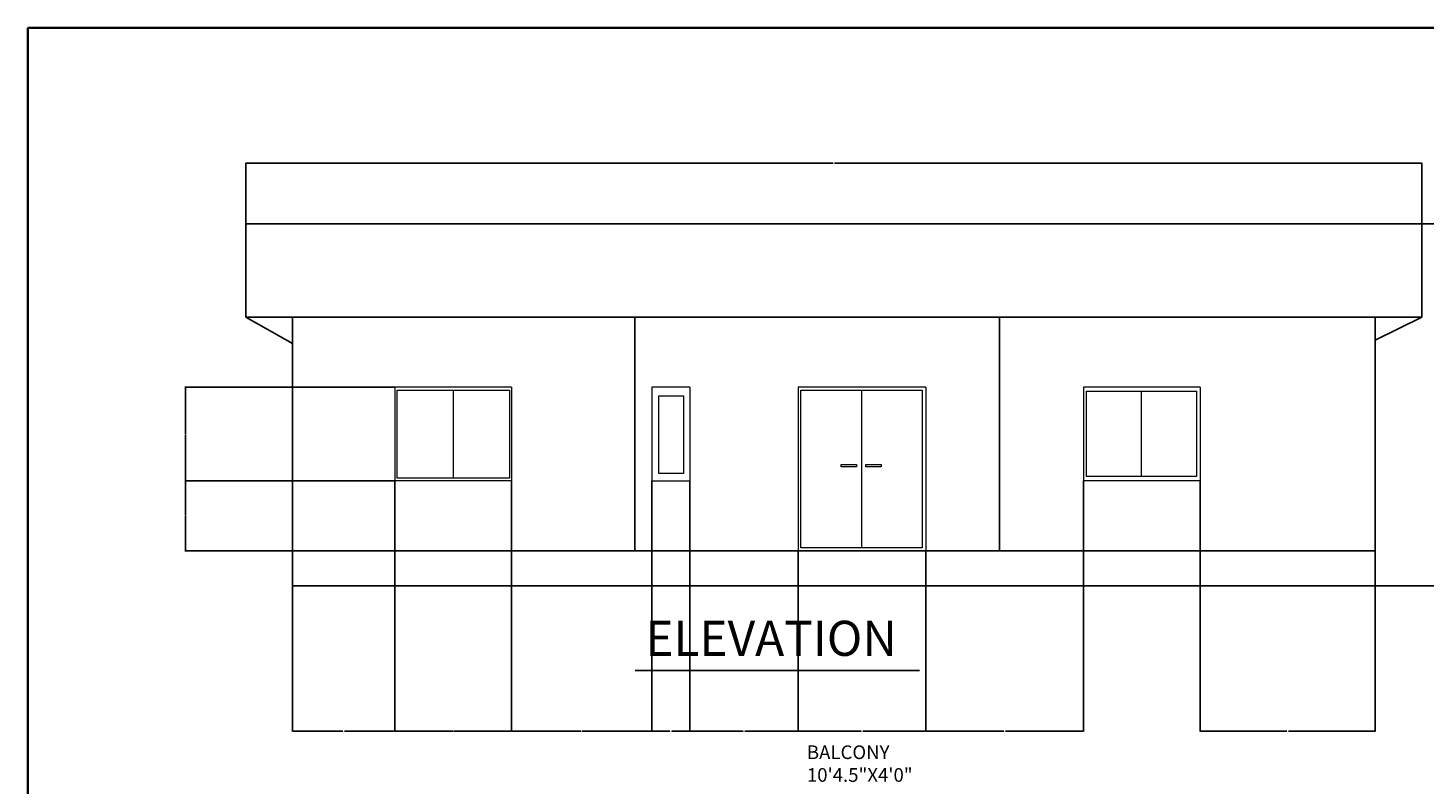
# Model space of a CAD drawing. Units: inches. Extents: x 2296 to 3812, y -1531 to 2564.
# Tile 5 of 10: x 2296 to 3013, y 2176 to 2564. Entities that reach past the tile are written whole.
import ezdxf

# ---------------------------------------------------------------- set-up
doc = ezdxf.new("R2010")
doc.units = ezdxf.units.IN
for name, color, linetype, lineweight in [('A-ANNO-DIMS', 2, 'Continuous', 18), ('A-ANNO-TEXT', 7, 'Continuous', 25), ('A-ANNO-TTLB', 7, 'Continuous', 35), ('A-AREA-IDEN', 7, 'Continuous', 18), ('A-ELEV', 7, 'Continuous', 25), ('A-ELEV-OPEN', 4, 'Continuous', 18)]:
    doc.layers.add(name, color=color, linetype=linetype, lineweight=lineweight)
doc.styles.get("Standard").update_dxf_attribs({"font": 'arial.ttf'})
doc.dimstyles.get("Standard").update_dxf_attribs({"dimtxt": 0.18, "dimasz": 0.18, "dimexe": 0.18, "dimexo": 0.0625, "dimgap": 0.09, "dimtad": 0, "dimtih": 1, "dimtoh": 1, "dimdec": 4, "dimzin": 0, "dimdsep": 46, "dimtxsty": 'Standard', "dimcen": 0.09, "dimadec": 0, "dimazin": 0, "dimtfac": 1, "dimtdec": 4, "dimtofl": 0, "dimtmove": 0, "dimatfit": 3, "dimfxl": 1, "dimtolj": 1, "dimtzin": 0, "dimarcsym": 0})

# ---------------------------------------------------------------- blocks, each defined once
blk = doc.blocks.new('*D147')
at = {"layer": 'A-ANNO-DIMS', "color": 0, "lineweight": -2, "transparency": 16777216}
for p, q in [((2408.07, 2463.85), (2408.07, 2495.06)), ((2408.25, 2494.88), (2709.61, 2494.88)), ((3011.77, 2494.88), (2710.4, 2494.88)), ((3011.95, 2463.85), (3011.95, 2495.06))]:
    blk.add_line(p, q, dxfattribs=at)
at = {"layer": 'A-ANNO-DIMS', "color": 0, "transparency": 16777216}
for points in [[(2408.25, 2494.91), (2408.25, 2494.85), (2408.07, 2494.88)], [(3011.77, 2494.91), (3011.77, 2494.85), (3011.95, 2494.88)]]:
    blk.add_solid(points, dxfattribs=at)
at = {"layer": 'Defpoints', "color": 0, "transparency": 16777216}
for p in [(3011.95, 2494.88), (2408.07, 2463.78), (3011.95, 2463.78)]:
    blk.add_point(p, dxfattribs=at)
at = {"layer": 'A-ANNO-DIMS', "color": 0, "transparency": 16777216, "insert": (2710.01, 2494.88), "char_height": 0.18, "attachment_point": 5}
blk.add_mtext('\\A1;603.9', dxfattribs=at)
blk = doc.blocks.new('*D148')
at = {"layer": 'A-ANNO-DIMS', "color": 0, "lineweight": -2, "transparency": 16777216}
for p, q in [((3012.01, 2463.78), (3043.23, 2463.78)), ((3043.05, 2463.6), (3043.05, 2370.97)), ((3043.05, 2277.96), (3043.05, 2370.6)), ((2988.01, 2277.78), (3043.23, 2277.78))]:
    blk.add_line(p, q, dxfattribs=at)
at = {"layer": 'A-ANNO-DIMS', "color": 0, "transparency": 16777216}
for points in [[(3043.02, 2463.6), (3043.08, 2463.6), (3043.05, 2463.78)], [(3043.02, 2277.96), (3043.08, 2277.96), (3043.05, 2277.78)]]:
    blk.add_solid(points, dxfattribs=at)
at = {"layer": 'Defpoints', "color": 0, "transparency": 16777216}
for p in [(3011.95, 2463.78), (2987.95, 2277.78), (3043.05, 2277.78)]:
    blk.add_point(p, dxfattribs=at)
at = {"layer": 'A-ANNO-DIMS', "color": 0, "transparency": 16777216, "insert": (3043.05, 2370.78), "char_height": 0.18, "attachment_point": 5}
blk.add_mtext('\\A1;186', dxfattribs=at)
blk = doc.blocks.new('*D149')
at = {"layer": 'A-ANNO-DIMS', "color": 0, "lineweight": -2, "transparency": 16777216}
for p, q in [((2484.53, 2331.72), (2484.53, 2203.12)), ((2432.07, 2295.72), (2432.07, 2203.12)), ((2432.25, 2203.3), (2457.91, 2203.3)), ((2484.35, 2203.3), (2458.7, 2203.3))]:
    blk.add_line(p, q, dxfattribs=at)
at = {"layer": 'A-ANNO-DIMS', "color": 0, "transparency": 16777216}
for points in [[(2432.25, 2203.33), (2432.25, 2203.27), (2432.07, 2203.3)], [(2484.35, 2203.33), (2484.35, 2203.27), (2484.53, 2203.3)]]:
    blk.add_solid(points, dxfattribs=at)
at = {"layer": 'Defpoints', "color": 0, "transparency": 16777216}
for p in [(2484.53, 2331.78), (2432.07, 2295.78), (2484.53, 2203.3)]:
    blk.add_point(p, dxfattribs=at)
at = {"layer": 'A-ANNO-DIMS', "color": 0, "transparency": 16777216, "insert": (2458.3, 2203.3), "char_height": 0.18, "attachment_point": 5}
blk.add_mtext('\\A1;52.46', dxfattribs=at)
blk = doc.blocks.new('*D150')
at = {"layer": 'A-ANNO-DIMS', "color": 0, "lineweight": -2, "transparency": 16777216}
for p, q in [((2484.53, 2331.72), (2484.53, 2203.12)), ((2544.53, 2331.72), (2544.53, 2203.12)), ((2484.71, 2203.3), (2514.31, 2203.3)), ((2544.35, 2203.3), (2514.75, 2203.3))]:
    blk.add_line(p, q, dxfattribs=at)
at = {"layer": 'A-ANNO-DIMS', "color": 0, "transparency": 16777216}
for points in [[(2484.71, 2203.33), (2484.71, 2203.27), (2484.53, 2203.3)], [(2544.35, 2203.33), (2544.35, 2203.27), (2544.53, 2203.3)]]:
    blk.add_solid(points, dxfattribs=at)
at = {"layer": 'Defpoints', "color": 0, "transparency": 16777216}
for p in [(2484.53, 2331.78), (2544.53, 2331.78), (2544.53, 2203.3)]:
    blk.add_point(p, dxfattribs=at)
at = {"layer": 'A-ANNO-DIMS', "color": 0, "transparency": 16777216, "insert": (2514.53, 2203.3), "char_height": 0.18, "attachment_point": 5}
blk.add_mtext('\\A1;60', dxfattribs=at)
blk = doc.blocks.new('*D151')
at = {"layer": 'A-ANNO-DIMS', "color": 0, "lineweight": -2, "transparency": 16777216}
for p, q in [((2544.53, 2331.72), (2544.53, 2203.12)), ((2616.53, 2331.72), (2616.53, 2203.12)), ((2544.71, 2203.3), (2580.31, 2203.3)), ((2616.35, 2203.3), (2580.75, 2203.3))]:
    blk.add_line(p, q, dxfattribs=at)
at = {"layer": 'A-ANNO-DIMS', "color": 0, "transparency": 16777216}
for points in [[(2544.71, 2203.33), (2544.71, 2203.27), (2544.53, 2203.3)], [(2616.35, 2203.33), (2616.35, 2203.27), (2616.53, 2203.3)]]:
    blk.add_solid(points, dxfattribs=at)
at = {"layer": 'Defpoints', "color": 0, "transparency": 16777216}
for p in [(2544.53, 2331.78), (2616.53, 2331.78), (2616.53, 2203.3)]:
    blk.add_point(p, dxfattribs=at)
at = {"layer": 'A-ANNO-DIMS', "color": 0, "transparency": 16777216, "insert": (2580.53, 2203.3), "char_height": 0.18, "attachment_point": 5}
blk.add_mtext('\\A1;72', dxfattribs=at)
blk = doc.blocks.new('*D152')
at = {"layer": 'A-ANNO-DIMS', "color": 0, "lineweight": -2, "transparency": 16777216}
for p, q in [((2616.53, 2331.72), (2616.53, 2203.12)), ((2636.1, 2331.72), (2636.1, 2203.12)), ((2616.71, 2203.3), (2625.86, 2203.3)), ((2635.92, 2203.3), (2626.77, 2203.3))]:
    blk.add_line(p, q, dxfattribs=at)
at = {"layer": 'A-ANNO-DIMS', "color": 0, "transparency": 16777216}
for points in [[(2616.71, 2203.33), (2616.71, 2203.27), (2616.53, 2203.3)], [(2635.92, 2203.33), (2635.92, 2203.27), (2636.1, 2203.3)]]:
    blk.add_solid(points, dxfattribs=at)
at = {"layer": 'Defpoints', "color": 0, "transparency": 16777216}
for p in [(2616.53, 2331.78), (2636.1, 2331.78), (2636.1, 2203.3)]:
    blk.add_point(p, dxfattribs=at)
at = {"layer": 'A-ANNO-DIMS', "color": 0, "transparency": 16777216, "insert": (2626.31, 2203.3), "char_height": 0.18, "attachment_point": 5}
blk.add_mtext('\\A1;19.565', dxfattribs=at)
blk = doc.blocks.new('*D153')
at = {"layer": 'A-ANNO-DIMS', "color": 0, "lineweight": -2, "transparency": 16777216}
for p, q in [((2636.1, 2331.72), (2636.1, 2203.12)), ((2691.63, 2295.72), (2691.63, 2203.12)), ((2636.28, 2203.3), (2663.47, 2203.3)), ((2691.45, 2203.3), (2664.25, 2203.3))]:
    blk.add_line(p, q, dxfattribs=at)
at = {"layer": 'A-ANNO-DIMS', "color": 0, "transparency": 16777216}
for points in [[(2636.28, 2203.33), (2636.28, 2203.27), (2636.1, 2203.3)], [(2691.45, 2203.33), (2691.45, 2203.27), (2691.63, 2203.3)]]:
    blk.add_solid(points, dxfattribs=at)
at = {"layer": 'Defpoints', "color": 0, "transparency": 16777216}
for p in [(2636.1, 2331.78), (2691.63, 2295.78), (2691.63, 2203.3)]:
    blk.add_point(p, dxfattribs=at)
at = {"layer": 'A-ANNO-DIMS', "color": 0, "transparency": 16777216, "insert": (2663.86, 2203.3), "char_height": 0.18, "attachment_point": 5}
blk.add_mtext('\\A1;55.53', dxfattribs=at)
blk = doc.blocks.new('*D154')
at = {"layer": 'A-ANNO-DIMS', "color": 0, "lineweight": -2, "transparency": 16777216}
for p, q in [((2691.63, 2295.72), (2691.63, 2203.12)), ((2757.3, 2295.72), (2757.3, 2203.12)), ((2691.81, 2203.3), (2724.07, 2203.3)), ((2757.12, 2203.3), (2724.86, 2203.3))]:
    blk.add_line(p, q, dxfattribs=at)
at = {"layer": 'A-ANNO-DIMS', "color": 0, "transparency": 16777216}
for points in [[(2691.81, 2203.33), (2691.81, 2203.27), (2691.63, 2203.3)], [(2757.12, 2203.33), (2757.12, 2203.27), (2757.3, 2203.3)]]:
    blk.add_solid(points, dxfattribs=at)
at = {"layer": 'Defpoints', "color": 0, "transparency": 16777216}
for p in [(2691.63, 2295.78), (2757.3, 2295.78), (2757.3, 2203.3)]:
    blk.add_point(p, dxfattribs=at)
at = {"layer": 'A-ANNO-DIMS', "color": 0, "transparency": 16777216, "insert": (2724.46, 2203.3), "char_height": 0.18, "attachment_point": 5}
blk.add_mtext('\\A1;65.68', dxfattribs=at)
blk = doc.blocks.new('*D155')
at = {"layer": 'A-ANNO-DIMS', "color": 0, "lineweight": -2, "transparency": 16777216}
for p, q in [((2838.14, 2331.72), (2838.14, 2203.12)), ((2757.3, 2295.72), (2757.3, 2203.12)), ((2757.48, 2203.3), (2797.32, 2203.3)), ((2837.96, 2203.3), (2798.11, 2203.3))]:
    blk.add_line(p, q, dxfattribs=at)
at = {"layer": 'A-ANNO-DIMS', "color": 0, "transparency": 16777216}
for points in [[(2757.48, 2203.33), (2757.48, 2203.27), (2757.3, 2203.3)], [(2837.96, 2203.33), (2837.96, 2203.27), (2838.14, 2203.3)]]:
    blk.add_solid(points, dxfattribs=at)
at = {"layer": 'Defpoints', "color": 0, "transparency": 16777216}
for p in [(2838.14, 2331.78), (2757.3, 2295.78), (2838.14, 2203.3)]:
    blk.add_point(p, dxfattribs=at)
at = {"layer": 'A-ANNO-DIMS', "color": 0, "transparency": 16777216, "insert": (2797.72, 2203.3), "char_height": 0.18, "attachment_point": 5}
blk.add_mtext('\\A1;80.84', dxfattribs=at)
blk = doc.blocks.new('*D156')
at = {"layer": 'A-ANNO-DIMS', "color": 0, "lineweight": -2, "transparency": 16777216}
for p, q in [((2898.14, 2331.72), (2898.14, 2203.12)), ((2987.95, 2295.72), (2987.95, 2203.12)), ((2898.32, 2203.3), (2942.67, 2203.3)), ((2987.77, 2203.3), (2943.42, 2203.3))]:
    blk.add_line(p, q, dxfattribs=at)
at = {"layer": 'A-ANNO-DIMS', "color": 0, "transparency": 16777216}
for points in [[(2898.32, 2203.33), (2898.32, 2203.27), (2898.14, 2203.3)], [(2987.77, 2203.33), (2987.77, 2203.27), (2987.95, 2203.3)]]:
    blk.add_solid(points, dxfattribs=at)
at = {"layer": 'Defpoints', "color": 0, "transparency": 16777216}
for p in [(2898.14, 2331.78), (2987.95, 2295.78), (2987.95, 2203.3)]:
    blk.add_point(p, dxfattribs=at)
at = {"layer": 'A-ANNO-DIMS', "color": 0, "transparency": 16777216, "insert": (2943.04, 2203.3), "char_height": 0.18, "attachment_point": 5}
blk.add_mtext('\\A1;89.81', dxfattribs=at)
blk = doc.blocks.new('*D157')
at = {"layer": 'A-ANNO-DIMS', "color": 0, "lineweight": -2, "transparency": 16777216}
for p, q in [((2484.47, 2379.78), (2376.79, 2379.78)), ((2376.97, 2379.6), (2376.97, 2355.97)), ((2376.97, 2331.96), (2376.97, 2355.6)), ((2484.47, 2331.78), (2376.79, 2331.78))]:
    blk.add_line(p, q, dxfattribs=at)
at = {"layer": 'A-ANNO-DIMS', "color": 0, "transparency": 16777216}
for points in [[(2376.94, 2379.6), (2377, 2379.6), (2376.97, 2379.78)], [(2376.94, 2331.96), (2377, 2331.96), (2376.97, 2331.78)]]:
    blk.add_solid(points, dxfattribs=at)
at = {"layer": 'Defpoints', "color": 0, "transparency": 16777216}
for p in [(2376.97, 2379.78), (2484.53, 2379.78), (2484.53, 2331.78)]:
    blk.add_point(p, dxfattribs=at)
at = {"layer": 'A-ANNO-DIMS', "color": 0, "transparency": 16777216, "insert": (2376.97, 2355.78), "char_height": 0.18, "attachment_point": 5}
blk.add_mtext('\\A1;48', dxfattribs=at)
blk = doc.blocks.new('*D158')
at = {"layer": 'A-ANNO-DIMS', "color": 0, "lineweight": -2, "transparency": 16777216}
for p, q in [((2484.47, 2331.78), (2376.79, 2331.78)), ((2376.97, 2331.6), (2376.97, 2313.97)), ((2376.97, 2295.96), (2376.97, 2313.6)), ((2432.01, 2295.78), (2376.79, 2295.78))]:
    blk.add_line(p, q, dxfattribs=at)
at = {"layer": 'A-ANNO-DIMS', "color": 0, "transparency": 16777216}
for points in [[(2376.94, 2331.6), (2377, 2331.6), (2376.97, 2331.78)], [(2376.94, 2295.96), (2377, 2295.96), (2376.97, 2295.78)]]:
    blk.add_solid(points, dxfattribs=at)
at = {"layer": 'Defpoints', "color": 0, "transparency": 16777216}
for p in [(2376.97, 2331.78), (2484.53, 2331.78), (2432.07, 2295.78)]:
    blk.add_point(p, dxfattribs=at)
at = {"layer": 'A-ANNO-DIMS', "color": 0, "transparency": 16777216, "insert": (2376.97, 2313.78), "char_height": 0.18, "attachment_point": 5}
blk.add_mtext('\\A1;36', dxfattribs=at)

msp = doc.modelspace()

# ---------------------------------------------------------------- linework, layer by layer
at = {"layer": 'A-ANNO-TEXT'}
msp.add_line((2608.0536, 2234.4), (2754.021, 2234.4), dxfattribs=at)
at = {"layer": 'A-ANNO-TTLB'}
msp.add_lwpolyline([(2296.1257, 2564.2989), (3812.4193, 2564.2989), (3812.4193, 1124.0028), (2296.1257, 1124.0028)], close=True, dxfattribs=at)
at = {"layer": 'A-ELEV'}
for p, q in [((3011.9477, 2463.7848), (2408.0693, 2463.7848)), ((2408.0693, 2415.7848), (2408.0693, 2463.7848)), ((3011.9477, 2415.7848), (3011.9477, 2463.7848)), ((3011.9477, 2415.7848), (2408.0693, 2415.7848)), ((2408.0693, 2415.7848), (2432.0693, 2402.2973)), ((2432.0693, 2415.7848), (2432.0693, 2277.7848)), ((2607.7523, 2415.7848), (2607.7523, 2295.7848)), ((2795.0769, 2295.7848), (2795.0769, 2415.7848)), ((2987.9477, 2415.7848), (2987.9477, 2277.7848)), ((3011.9477, 2415.7848), (2987.9477, 2404.011)), ((2987.9477, 2295.7848), (2432.0693, 2295.7848)), ((2987.9477, 2277.7848), (2432.0693, 2277.7848))]:
    msp.add_line(p, q, dxfattribs=at)
at = {"layer": 'A-ELEV-OPEN'}
for p, q in [((2484.5339, 2379.7848), (2484.5339, 2331.7848)), ((2544.5339, 2379.7848), (2484.5339, 2379.7848)), ((2514.5665, 2378.3619), (2514.5665, 2333.0987)), ((2544.5339, 2379.7848), (2544.5339, 2331.7848)), ((2616.5304, 2379.7848), (2616.5304, 2331.7848)), ((2616.5304, 2379.7848), (2616.5304, 2331.7848)), ((2636.0952, 2379.7848), (2616.5304, 2379.7848)), ((2636.0952, 2379.7848), (2636.0952, 2331.7848)), ((2691.6251, 2379.7848), (2691.6251, 2295.7848)), ((2757.3002, 2379.7848), (2691.6251, 2379.7848)), ((2724.2236, 2378.2317), (2724.2236, 2297.4307)), ((2757.3002, 2379.7848), (2757.3002, 2295.7848)), ((2838.1353, 2379.7848), (2838.1353, 2331.7848)), ((2898.1353, 2379.7848), (2838.1353, 2379.7848)), ((2868.0536, 2333.9785), (2868.0536, 2377.7429)), ((2898.1353, 2379.7848), (2898.1353, 2331.7848)), ((2544.5339, 2331.7848), (2484.5339, 2331.7848)), ((2616.5304, 2331.7848), (2636.0952, 2331.7848)), ((2898.1353, 2331.7848), (2838.1353, 2331.7848))]:
    msp.add_line(p, q, dxfattribs=at)
for points in [[(2485.6766, 2378.3619), (2543.4563, 2378.3619), (2543.4563, 2333.0987), (2485.6766, 2333.0987)], [(2620.1507, 2375.4456), (2632.8249, 2375.4456), (2632.8249, 2335.4646), (2620.1507, 2335.4646)], [(2693.1051, 2378.2317), (2755.3422, 2378.2317), (2755.3422, 2297.4307), (2693.1051, 2297.4307)], [(2839.8095, 2377.7429), (2896.2977, 2377.7429), (2896.2977, 2333.9785), (2839.8095, 2333.9785)], [(2713.7463, 2340.2085), (2721.5628, 2340.2085), (2721.5628, 2339.0064), (2713.7463, 2339.0064)], [(2726.4292, 2340.2085), (2734.2456, 2340.2085), (2734.2456, 2339.0064), (2726.4292, 2339.0064)]]:
    msp.add_lwpolyline(points, close=True, dxfattribs=at)

# ---------------------------------------------------------------- texts
at = {"layer": 'A-ANNO-TEXT', "insert": (2613.2037, 2259.9039), "char_height": 18, "attachment_point": 1}
msp.add_mtext_dynamic_manual_height_columns('ELEVATION', width=329.824126, gutter_width=12.5, heights=[0], dxfattribs=at)
at = {"layer": 'A-AREA-IDEN', "insert": (2696.1698, 2195.9097), "char_height": 7, "attachment_point": 1}
msp.add_mtext_dynamic_manual_height_columns('BALCONY\\P10\'4.5"X4\'0"', width=74.273028, gutter_width=12.5, heights=[0], dxfattribs=at)

# ---------------------------------------------------------------- dimensions: what is measured, and where the dimension line sits
at = {"layer": 'A-ANNO-DIMS'}
for base, p1, p2, override, picture, middle in [((3011.9477, 2494.8848), (2408.0693, 2463.7848), (3011.9477, 2463.7848), {"dimdec": 1, "dimlfac": 1, "dimrnd": 0, "dimzin": 0, "dimdsep": 46, "dimlunit": 2}, '*D147', (2710.0085, 2494.8848)), ((2484.5339, 2203.3), (2432.0693, 2295.7848), (2484.5339, 2331.7848), {"dimdec": 2, "dimlfac": 1, "dimrnd": 0, "dimzin": 0, "dimdsep": 46, "dimlunit": 2}, '*D149', (2458.3016, 2203.3)), ((2544.5339, 2203.3), (2484.5339, 2331.7848), (2544.5339, 2331.7848), {"dimdec": 0, "dimlfac": 1, "dimrnd": 0, "dimzin": 0, "dimdsep": 46, "dimlunit": 2}, '*D150', (2514.5339, 2203.3)), ((2616.5304, 2203.3), (2544.5339, 2331.7848), (2616.5304, 2331.7848), {"dimdec": 0, "dimlfac": 1, "dimrnd": 0, "dimzin": 0, "dimdsep": 46, "dimlunit": 2}, '*D151', (2580.5321, 2203.3)), ((2636.0952, 2203.3), (2616.5304, 2331.7848), (2636.0952, 2331.7848), {"dimdec": 3, "dimlfac": 1, "dimrnd": 0, "dimzin": 0, "dimdsep": 46, "dimlunit": 2}, '*D152', (2626.3128, 2203.3)), ((2691.6251, 2203.3), (2636.0952, 2331.7848), (2691.6251, 2295.7848), {"dimdec": 2, "dimlfac": 1, "dimrnd": 0, "dimzin": 0, "dimdsep": 46, "dimlunit": 2}, '*D153', (2663.8602, 2203.3)), ((2838.1353, 2203.3), (2757.3002, 2295.7848), (2838.1353, 2331.7848), {"dimdec": 2, "dimlfac": 1, "dimrnd": 0, "dimzin": 0, "dimdsep": 46, "dimlunit": 2}, '*D155', (2797.7177, 2203.3)), ((2987.9477, 2203.3), (2898.1353, 2331.7848), (2987.9477, 2295.7848), {"dimdec": 2, "dimlfac": 1, "dimrnd": 0, "dimzin": 0, "dimdsep": 46, "dimlunit": 2}, '*D156', (2943.0415, 2203.3)), ((2757.3002, 2203.3), (2691.6251, 2295.7848), (2757.3002, 2295.7848), {"dimdec": 2, "dimlfac": 1, "dimrnd": 0, "dimzin": 0, "dimdsep": 46, "dimlunit": 2}, '*D154', (2724.4626, 2203.3))]:
    dim = msp.add_linear_dim(base=base, p1=p1, p2=p2, dimstyle='Standard', override=override, dxfattribs=at)
    dim.commit()
    dim.dimension.update_dxf_attribs({"geometry": picture, "text_midpoint": middle})
for base, p1, p2, picture, middle in [((3043.0477, 2277.7848), (3011.9477, 2463.7848), (2987.9477, 2277.7848), '*D148', (3043.0477, 2370.7848)), ((2376.9693, 2379.7848), (2484.5339, 2331.7848), (2484.5339, 2379.7848), '*D157', (2376.9693, 2355.7848)), ((2376.9693, 2331.7848), (2432.0693, 2295.7848), (2484.5339, 2331.7848), '*D158', (2376.9693, 2313.7848))]:
    dim = msp.add_linear_dim(base=base, p1=p1, p2=p2, angle=90, dimstyle='Standard', override={"dimdec": 0, "dimlfac": 1, "dimrnd": 0, "dimzin": 0, "dimdsep": 46, "dimlunit": 2}, dxfattribs=at)
    dim.commit()
    dim.dimension.update_dxf_attribs({"geometry": picture, "text_midpoint": middle})

doc.saveas('drawing.dxf')
